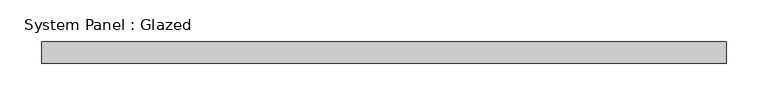
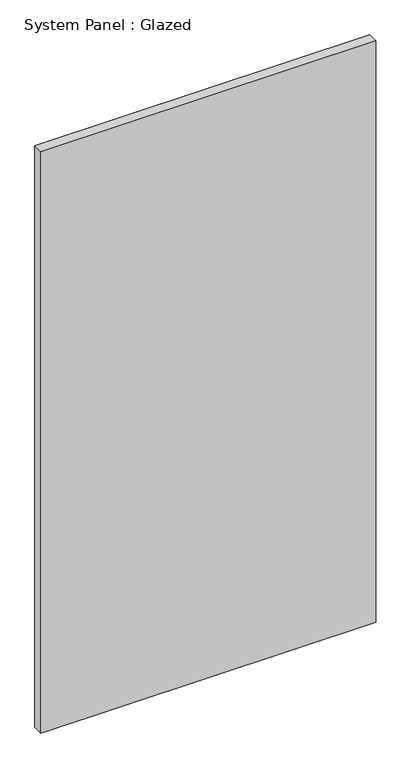
"""IFC4 building model written with IfcOpenShell, lengths in millimetres: plate geometry, System Panel : Glazed."""

from ifc_helpers import new_model, si_unit, origin, origin_with_axes, place, context, project, spatial, polyline, outline, extrude, source, transform, mapped, element, save


def system_panel_glazed_affe7bbf(model_context):
    return source(origin(), model_context, "Body", "SweptSolid", [
        extrude(outline(polyline([(409.575, 19.05), (-409.575, 19.05), (-409.575, 44.45), (409.575, 44.45), (409.575, 19.05)])), origin_with_axes(), (0.0, 0.0, 1.0), 1502.9147167),
    ])


if __name__ == "__main__":
    model = new_model("IFC4")
    model_context = context("Model", 3, world=origin())
    ifc_project = project(units=[si_unit("LENGTHUNIT", "METRE", prefix="MILLI")], contexts=[model_context])
    site = spatial("IfcSite", under=ifc_project)
    building = spatial("IfcBuilding", under=site)
    placement = place(None, origin())
    system_panel_glazed_shape = system_panel_glazed_affe7bbf(model_context)
    element("IfcPlate", 1, ObjectType="System Panel : Glazed", at=placement, inside=building, context=model_context, shape_type="MappedRepresentation", body=[
        mapped(system_panel_glazed_shape, transform((0.0, 0.0, 0.0), x_axis=(1.0, 0.0, 0.0), y_axis=(0.0, 1.0, 0.0), z_axis=(0.0, 0.0, 1.0))),
    ])
    save(model, "model.ifc")

# Revit data of these elements
# Type "System Panel : Glazed"
#   Construction Type Id = "GSP4R"
#   Analytic Construction = "1/8 in Pilkington single glazing"
#   Visual Light Transmittance = 0.9
#   Solar Heat Gain Coefficient = 0.86
#   Heat Transfer Coefficient (U) = 1.18115 BTU/(h·ft²·°F)
#   Define Thermal Properties by = 1
# Element 1 (IfcPlate, "System Panel : Glazed")
#   Materials on its faces: "Glass"
# Materials
#   "Glass": class "Glass", colour RGB 0 128 192, transparency 0.75, Description = "Soda Lime Glass", Cost = 0
